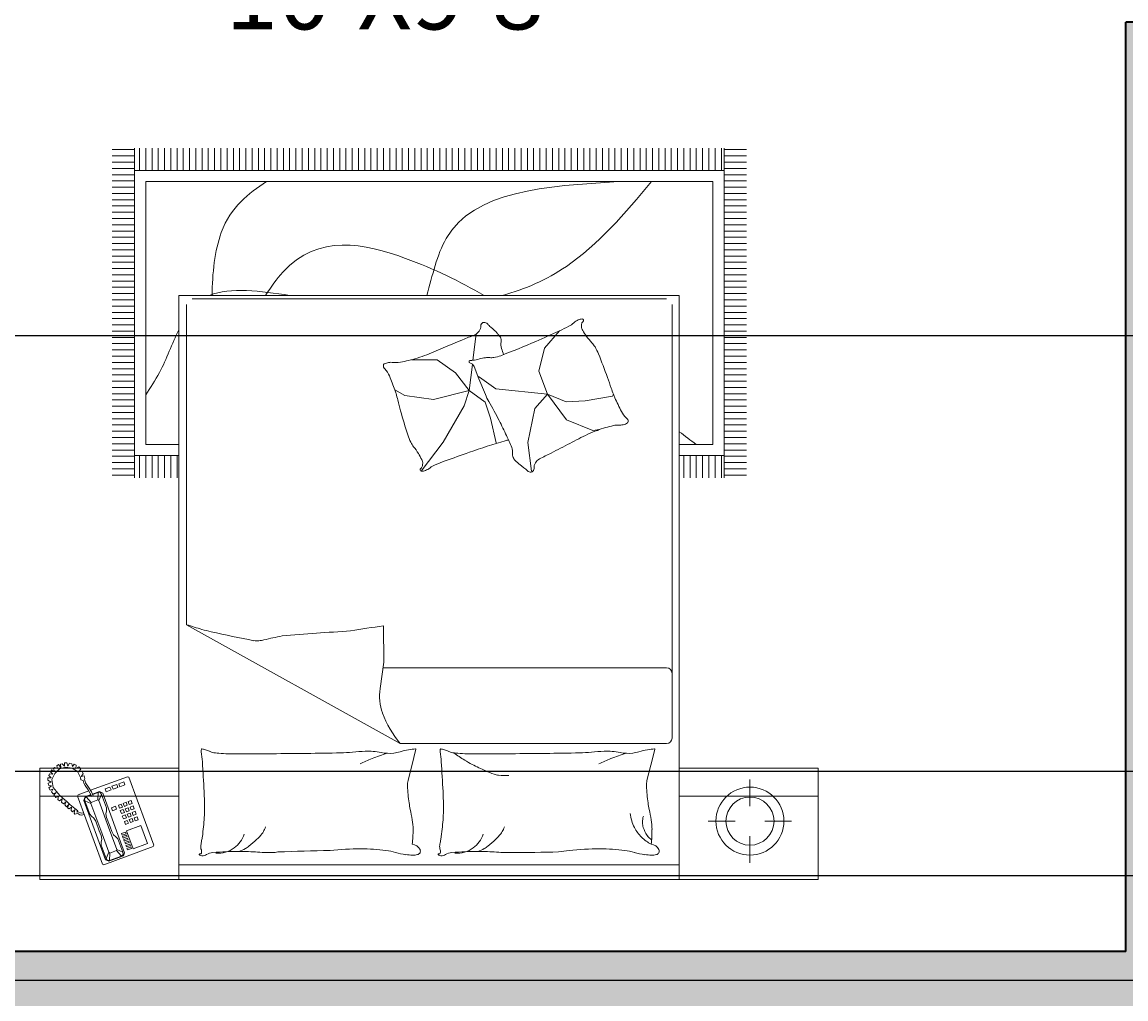
# Model space of a CAD drawing. Units: inches. Extents: x 311 to 815, y -527 to 136.
# Tile 8 of 21: x 444 to 539, y -294 to -210. Entities that reach past the tile are written whole.
import ezdxf

# ---------------------------------------------------------------- set-up
doc = ezdxf.new("R2010")
doc.units = ezdxf.units.IN
doc.header["$MEASUREMENT"] = 0
for name, color, linetype, lineweight in [('A-ANNO-DIMS', 1, 'Continuous', 18), ('A-AREA-IDEN', 8, 'Continuous', 18), ('A-WALL-PATT', 242, 'Continuous', 13), ('wall', 1, 'Continuous', 35)]:
    doc.layers.add(name, color=color, linetype=linetype, lineweight=lineweight)
doc.layers.add('furniture', color=50, linetype='Continuous', lineweight=13, transparency=0.8)
doc.styles.add('DIM_FONT', font='SIMPLEX.shx', dxfattribs={"width": 0.8})
doc.styles.get("Standard").update_dxf_attribs({"font": 'arial.ttf'})
doc.dimstyles.get("Standard").update_dxf_attribs({"dimtxt": 0.18, "dimasz": 0.18, "dimexe": 0.18, "dimexo": 0.0625, "dimgap": 0.09, "dimtad": 0, "dimtih": 1, "dimtoh": 1, "dimdec": 1, "dimzin": 0, "dimdsep": 46, "dimlunit": 4, "dimtxsty": 'Standard', "dimcen": 0.09, "dimadec": 0, "dimazin": 0, "dimtfac": 1, "dimtdec": 1, "dimtofl": 0, "dimtmove": 0, "dimatfit": 3, "dimfxl": 1, "dimtolj": 1, "dimtzin": 0, "dimarcsym": 0})

# ---------------------------------------------------------------- blocks, each defined once
blk = doc.blocks.new('A$C4F634EDD')
for p, q in [((0, 2.6295), (0, 2.2295)), ((0.5, 2.6295), (0, 2.6295)), ((0.5, 2.6295), (2.3, 2.6295)), ((0.5, 0.5295), (0.5, 2.6295)), ((0.5, 2.2295), (0.5, 2.6295)), ((2.3, 2.6295), (2.3, 0.5295)), ((2.3, 2.6295), (2.8, 2.6295)), ((2.3, 2.2295), (2.3, 2.6295)), ((2.8, 2.6295), (2.8, 2.2295)), ((0.2457, 2.5697), (0.2457, 2.4733)), ((0.5, 2.5771), (2.3, 2.5771)), ((2.392, 2.5115), (2.5692, 2.5765)), ((2.4946, 2.5331), (2.4985, 2.5445)), ((2.4985, 2.5445), (2.5516, 2.564)), ((2.5062, 2.5454), (2.5004, 2.5392)), ((2.5062, 2.5454), (2.5487, 2.561)), ((2.5235, 2.5256), (2.5062, 2.5454)), ((2.5483, 2.5347), (2.5487, 2.561)), ((2.5487, 2.561), (2.5571, 2.56)), ((2.5615, 2.5536), (2.5514, 2.5318)), ((2.5516, 2.564), (2.5637, 2.5584)), ((2.5571, 2.56), (2.5615, 2.5536)), ((2.5615, 2.5536), (2.5791, 2.5058)), ((2.5637, 2.5584), (2.6418, 2.3458)), ((2.5692, 2.5765), (2.574, 2.5743)), ((2.574, 2.5743), (2.6638, 2.3298)), ((2.3898, 2.5066), (2.392, 2.5115)), ((2.4795, 2.2621), (2.3898, 2.5066)), ((2.412, 2.5007), (2.4634, 2.5196)), ((2.4634, 2.5196), (2.4875, 2.454)), ((2.4842, 2.5232), (2.47, 2.518)), ((2.47, 2.518), (2.472, 2.5127)), ((2.472, 2.5127), (2.4862, 2.5179)), ((2.4881, 2.5126), (2.4739, 2.5074)), ((2.4739, 2.5074), (2.4759, 2.502)), ((2.4759, 2.502), (2.4901, 2.5073)), ((2.492, 2.5019), (2.4778, 2.4967)), ((2.4862, 2.5179), (2.4842, 2.5232)), ((2.4901, 2.5073), (2.4881, 2.5126)), ((2.494, 2.4966), (2.492, 2.5019)), ((2.5734, 2.3187), (2.4946, 2.5331)), ((2.5004, 2.5392), (2.5013, 2.5315)), ((2.5013, 2.5315), (2.5188, 2.4836)), ((2.5013, 2.5315), (2.5231, 2.5214)), ((2.5231, 2.5214), (2.5235, 2.5256)), ((2.5523, 2.4417), (2.5231, 2.5214)), ((2.5483, 2.5347), (2.5235, 2.5256)), ((2.5514, 2.5318), (2.5483, 2.5347)), ((2.5807, 2.4521), (2.5514, 2.5318)), ((2.5791, 2.5058), (2.5788, 2.4956)), ((2.4361, 2.4352), (2.412, 2.5007)), ((2.4778, 2.4967), (2.4798, 2.4914)), ((2.4798, 2.4914), (2.494, 2.4966)), ((2.4959, 2.4913), (2.4817, 2.4861)), ((2.4817, 2.4861), (2.4837, 2.4808)), ((2.4837, 2.4808), (2.4979, 2.486)), ((2.4998, 2.4807), (2.4856, 2.4755)), ((2.4856, 2.4755), (2.4876, 2.4702)), ((2.4876, 2.4702), (2.5018, 2.4754)), ((2.5037, 2.47), (2.4895, 2.4648)), ((2.4895, 2.4648), (2.4915, 2.4595)), ((2.4915, 2.4595), (2.5057, 2.4647)), ((2.4979, 2.486), (2.4959, 2.4913)), ((2.5018, 2.4754), (2.4998, 2.4807)), ((2.5057, 2.4647), (2.5037, 2.47)), ((2.5188, 2.4836), (2.5256, 2.4761)), ((2.5256, 2.4761), (2.5342, 2.4692)), ((2.5342, 2.4692), (2.5405, 2.4574)), ((2.5788, 2.4956), (2.5767, 2.4848)), ((2.5767, 2.4848), (2.5795, 2.4717)), ((2.5795, 2.4717), (2.586, 2.454)), ((2.4875, 2.454), (2.4361, 2.4352)), ((2.4634, 2.4211), (2.474, 2.425)), ((2.474, 2.425), (2.4779, 2.4143)), ((2.4811, 2.4276), (2.4917, 2.4315)), ((2.485, 2.4169), (2.4811, 2.4276)), ((2.4917, 2.4315), (2.4956, 2.4208)), ((2.5405, 2.4574), (2.547, 2.4397)), ((2.5594, 2.4061), (2.547, 2.4397)), ((2.5523, 2.4417), (2.5875, 2.346)), ((2.5807, 2.4521), (2.6158, 2.3564)), ((2.5984, 2.4204), (2.586, 2.454)), ((0.0957, 2.4197), (0.192, 2.4197)), ((0.2994, 2.4197), (0.3957, 2.4197)), ((2.4457, 2.4146), (2.4563, 2.4185)), ((2.4496, 2.4039), (2.4457, 2.4146)), ((2.4602, 2.4078), (2.4496, 2.4039)), ((2.4528, 2.3951), (2.4635, 2.399)), ((2.4567, 2.3844), (2.4528, 2.3951)), ((2.4563, 2.4185), (2.4602, 2.4078)), ((2.4674, 2.3883), (2.4567, 2.3844)), ((2.4673, 2.4104), (2.4634, 2.4211)), ((2.4635, 2.399), (2.4674, 2.3883)), ((2.4779, 2.4143), (2.4673, 2.4104)), ((2.4706, 2.4016), (2.4812, 2.4055)), ((2.4745, 2.3909), (2.4706, 2.4016)), ((2.4851, 2.3949), (2.4745, 2.3909)), ((2.4777, 2.3821), (2.4883, 2.386)), ((2.4816, 2.3715), (2.4777, 2.3821)), ((2.4812, 2.4055), (2.4851, 2.3949)), ((2.4956, 2.4208), (2.485, 2.4169)), ((2.4883, 2.4081), (2.4989, 2.412)), ((2.4922, 2.3975), (2.4883, 2.4081)), ((2.4883, 2.386), (2.4922, 2.3754)), ((2.5028, 2.4014), (2.4922, 2.3975)), ((2.4954, 2.3886), (2.5061, 2.3925)), ((2.4993, 2.378), (2.4954, 2.3886)), ((2.4989, 2.412), (2.5028, 2.4014)), ((2.51, 2.3819), (2.4993, 2.378)), ((2.5061, 2.3925), (2.51, 2.3819)), ((2.5238, 2.3769), (2.538, 2.3821)), ((2.538, 2.3821), (2.5419, 2.3715)), ((2.5622, 2.393), (2.5594, 2.4061)), ((2.5598, 2.372), (2.5601, 2.3822)), ((2.5601, 2.3822), (2.5622, 2.393)), ((2.6047, 2.4086), (2.5984, 2.4204)), ((2.6133, 2.4017), (2.6047, 2.4086)), ((2.6201, 2.3941), (2.6133, 2.4017)), ((2.6376, 2.3463), (2.6201, 2.3941)), ((2.6499, 2.3979), (2.6397, 2.3953)), ((2.6417, 2.39), (2.6488, 2.391)), ((2.6488, 2.391), (2.6538, 2.3895)), ((2.6551, 2.397), (2.6499, 2.3979)), ((2.6538, 2.3895), (2.6596, 2.388)), ((2.6627, 2.392), (2.6551, 2.397)), ((2.6596, 2.388), (2.6626, 2.3867)), ((2.6626, 2.3867), (2.6662, 2.388)), ((2.6692, 2.394), (2.6627, 2.392)), ((2.6662, 2.388), (2.6632, 2.3828)), ((2.6632, 2.3828), (2.6736, 2.3744)), ((2.6736, 2.3944), (2.6692, 2.394)), ((2.6765, 2.391), (2.6736, 2.3944)), ((2.6742, 2.3795), (2.6765, 2.391)), ((2.6824, 2.3858), (2.6742, 2.3795)), ((2.6873, 2.3815), (2.6824, 2.3858)), ((0.2457, 2.366), (0.2457, 2.2697)), ((2.46, 2.3756), (2.4706, 2.3795)), ((2.4639, 2.365), (2.46, 2.3756)), ((2.4745, 2.3689), (2.4639, 2.365)), ((2.4672, 2.3561), (2.4778, 2.36)), ((2.4711, 2.3455), (2.4672, 2.3561)), ((2.4706, 2.3795), (2.4745, 2.3689)), ((2.4817, 2.3494), (2.4711, 2.3455)), ((2.4778, 2.36), (2.4817, 2.3494)), ((2.4922, 2.3754), (2.4816, 2.3715)), ((2.4849, 2.3626), (2.4955, 2.3665)), ((2.4888, 2.352), (2.4849, 2.3626)), ((2.4994, 2.3559), (2.4888, 2.352)), ((2.4955, 2.3665), (2.4994, 2.3559)), ((2.5026, 2.3691), (2.5132, 2.373)), ((2.5065, 2.3585), (2.5026, 2.3691)), ((2.5171, 2.3624), (2.5065, 2.3585)), ((2.5132, 2.373), (2.5171, 2.3624)), ((2.5277, 2.3663), (2.5238, 2.3769)), ((2.5419, 2.3715), (2.5277, 2.3663)), ((2.5774, 2.3242), (2.5598, 2.372)), ((2.5774, 2.3242), (2.5875, 2.346)), ((2.5875, 2.346), (2.5905, 2.3431)), ((2.5905, 2.3431), (2.5901, 2.3168)), ((2.6154, 2.3522), (2.5905, 2.3431)), ((2.6158, 2.3564), (2.6154, 2.3522)), ((2.6154, 2.3522), (2.6327, 2.3324)), ((2.6376, 2.3463), (2.6158, 2.3564)), ((2.6418, 2.3458), (2.6369, 2.332)), ((2.6385, 2.3386), (2.6376, 2.3463)), ((2.6736, 2.3744), (2.6922, 2.3593)), ((2.6853, 2.369), (2.6873, 2.3815)), ((2.6946, 2.376), (2.6853, 2.369)), ((2.6922, 2.3593), (2.7051, 2.3473)), ((2.6995, 2.3713), (2.6946, 2.376)), ((2.695, 2.3603), (2.6995, 2.3713)), ((2.7031, 2.3682), (2.695, 2.3603)), ((2.7096, 2.3616), (2.7031, 2.3682)), ((2.7051, 2.3473), (2.7079, 2.3475)), ((2.7062, 2.351), (2.7096, 2.3616)), ((2.7147, 2.3578), (2.7062, 2.351)), ((2.7079, 2.3475), (2.7079, 2.3443)), ((2.7079, 2.3443), (2.727, 2.3277)), ((2.7214, 2.3517), (2.7147, 2.3578)), ((2.7196, 2.34), (2.7214, 2.3517)), ((2.7286, 2.3466), (2.7196, 2.34)), ((2.7346, 2.3423), (2.7286, 2.3466)), ((2.732, 2.3295), (2.7346, 2.3423)), ((0, 2.3301), (0.5, 2.3301)), ((2.8, 2.3301), (2.3, 2.3301)), ((2.6172, 2.3086), (2.4844, 2.2599)), ((2.5362, 2.305), (2.5185, 2.2985)), ((2.5401, 2.2944), (2.5362, 2.305)), ((2.561, 2.3141), (2.5433, 2.3076)), ((2.5433, 2.3076), (2.5472, 2.297)), ((2.5472, 2.297), (2.5649, 2.3035)), ((2.5649, 2.3035), (2.561, 2.3141)), ((2.5855, 2.3131), (2.5734, 2.3187)), ((2.5818, 2.3178), (2.5774, 2.3242)), ((2.5901, 2.3168), (2.5818, 2.3178)), ((2.6104, 2.3222), (2.5855, 2.3131)), ((2.5901, 2.3168), (2.6097, 2.324)), ((2.613, 2.3312), (2.6077, 2.3293)), ((2.6077, 2.3293), (2.6135, 2.3141)), ((2.6192, 2.3174), (2.613, 2.3312)), ((2.6135, 2.3141), (2.6244, 2.2977)), ((2.6153, 2.3261), (2.6327, 2.3324)), ((2.6369, 2.332), (2.6161, 2.3243)), ((2.626, 2.3069), (2.6192, 2.3174)), ((2.6616, 2.3249), (2.6234, 2.3109)), ((2.6365, 2.2916), (2.626, 2.3069)), ((2.6327, 2.3324), (2.6385, 2.3386)), ((2.6638, 2.3298), (2.6616, 2.3249)), ((2.727, 2.3277), (2.7512, 2.2983)), ((2.7423, 2.3345), (2.732, 2.3295)), ((2.7406, 2.3172), (2.7495, 2.325)), ((2.7519, 2.3218), (2.7406, 2.3172)), ((2.7495, 2.325), (2.7423, 2.3345)), ((2.7575, 2.3144), (2.7519, 2.3218)), ((2.7526, 2.3045), (2.7575, 2.3144)), ((2.7622, 2.308), (2.7526, 2.3045)), ((2.7673, 2.2997), (2.7622, 2.308)), ((0.5953, 2.1912), (0.616, 2.2738)), ((1.4546, 2.1912), (1.4752, 2.2738)), ((2.5114, 2.2959), (2.4936, 2.2894)), ((2.4936, 2.2894), (2.4976, 2.2788)), ((2.4976, 2.2788), (2.5153, 2.2853)), ((2.5153, 2.2853), (2.5114, 2.2959)), ((2.5185, 2.2985), (2.5224, 2.2879)), ((2.5224, 2.2879), (2.5401, 2.2944)), ((2.6244, 2.2977), (2.6349, 2.2825)), ((2.6349, 2.2825), (2.638, 2.273)), ((2.6407, 2.2834), (2.6365, 2.2916)), ((2.6399, 2.2712), (2.6374, 2.2659)), ((2.6374, 2.2659), (2.6398, 2.257)), ((2.638, 2.273), (2.6399, 2.2712)), ((2.6438, 2.2739), (2.6407, 2.2834)), ((2.6519, 2.2716), (2.6438, 2.2739)), ((2.6535, 2.2628), (2.6519, 2.2716)), ((2.6636, 2.2409), (2.6535, 2.2628)), ((2.756, 2.2695), (2.7459, 2.2483)), ((2.7512, 2.2983), (2.756, 2.2695)), ((2.7574, 2.2924), (2.7673, 2.2997)), ((2.7687, 2.2905), (2.7574, 2.2924)), ((2.7587, 2.279), (2.7699, 2.2828)), ((2.7708, 2.2725), (2.7587, 2.279)), ((2.759, 2.2637), (2.7706, 2.2643)), ((2.7676, 2.2559), (2.759, 2.2637)), ((2.7699, 2.2828), (2.7687, 2.2905)), ((2.7706, 2.2643), (2.7708, 2.2725)), ((0, 2.2295), (0.5, 2.2295)), ((2.8, 2.2295), (2.3, 2.2295)), ((2.4844, 2.2599), (2.4795, 2.2621)), ((2.6398, 2.257), (2.6509, 2.259)), ((2.6509, 2.259), (2.6431, 2.2492)), ((2.6431, 2.2492), (2.6473, 2.2398)), ((2.6473, 2.2398), (2.6592, 2.2429)), ((2.6592, 2.2429), (2.6521, 2.2314)), ((2.6521, 2.2314), (2.6598, 2.2248)), ((2.6598, 2.2248), (2.6697, 2.2309)), ((2.6836, 2.2287), (2.6636, 2.2409)), ((2.6697, 2.2309), (2.6684, 2.219)), ((2.6761, 2.2145), (2.6821, 2.2237)), ((2.6821, 2.2237), (2.6843, 2.2135)), ((2.7063, 2.2256), (2.6836, 2.2287)), ((2.7284, 2.2317), (2.7063, 2.2256)), ((2.7255, 2.2152), (2.7242, 2.2265)), ((2.7242, 2.2265), (2.7324, 2.2165)), ((2.7459, 2.2483), (2.7284, 2.2317)), ((2.7386, 2.2208), (2.7354, 2.2306)), ((2.7354, 2.2306), (2.7462, 2.2264)), ((2.7509, 2.2314), (2.7459, 2.2418)), ((2.7459, 2.2418), (2.7568, 2.2352)), ((2.7462, 2.2264), (2.7509, 2.2314)), ((2.7529, 2.2505), (2.7645, 2.2498)), ((2.7607, 2.2424), (2.7529, 2.2505)), ((2.7568, 2.2352), (2.7607, 2.2424)), ((2.7645, 2.2498), (2.7676, 2.2559)), ((0.5878, 2.1612), (0.5953, 2.1912)), ((1.4471, 2.1612), (1.4546, 2.1912)), ((2.6684, 2.219), (2.6761, 2.2145)), ((2.6843, 2.2135), (2.6927, 2.2117)), ((2.6927, 2.2117), (2.6986, 2.222)), ((2.6986, 2.222), (2.7019, 2.2098)), ((2.7019, 2.2098), (2.7102, 2.2104)), ((2.7102, 2.2104), (2.7113, 2.2218)), ((2.7113, 2.2218), (2.7192, 2.2137)), ((2.7192, 2.2137), (2.7255, 2.2152)), ((2.7324, 2.2165), (2.7386, 2.2208)), ((0.5258, 2.121), (0.5258, 0.5617)), ((1.5035, 2.141), (0.5458, 2.141)), ((1.5035, 2.141), (2.2716, 1.7136)), ((1.576, 1.9433), (1.5624, 1.8479)), ((0.5458, 1.8684), (1.5653, 1.8684)), ((1.5624, 1.8479), (1.5641, 1.7178)), ((2.2716, 0.5617), (2.2716, 1.7136)), ((0.2586, 1.1753), (0.3386, 1.1753)), ((0.2586, 1.1528), (0.3386, 1.1528)), ((0.3386, 0), (0.3386, 1.1852)), ((0.3486, 1.1052), (0.3486, 1.1852)), ((0.3711, 1.1052), (0.3711, 1.1852)), ((0.3936, 1.1052), (0.3936, 1.1852)), ((0.4161, 1.1052), (0.4161, 1.1852)), ((0.4386, 1.1052), (0.4386, 1.1852)), ((0.4611, 1.1052), (0.4611, 1.1852)), ((0.4836, 1.1052), (0.4836, 1.1852)), ((1.031, 1.1612), (1.0448, 1.0581)), ((1.4276, 1.1611), (1.3484, 1.0571)), ((2.3061, 1.1052), (2.3061, 1.1852)), ((2.3286, 1.1052), (2.3286, 1.1852)), ((2.3511, 1.1052), (2.3511, 1.1852)), ((2.3736, 1.1052), (2.3736, 1.1852)), ((2.3961, 1.1052), (2.3961, 1.1852)), ((2.4186, 1.1052), (2.4186, 1.1852)), ((2.4411, 1.1052), (2.4411, 1.1852)), ((2.4588, 1.1852), (2.4588, 0)), ((2.4588, 1.1753), (2.5388, 1.1753)), ((2.4588, 1.1528), (2.5388, 1.1528)), ((0.2586, 1.1303), (0.3386, 1.1303)), ((2.4588, 1.1303), (2.5388, 1.1303)), ((0.2586, 1.1078), (0.3386, 1.1078)), ((0.2586, 1.0853), (0.3386, 1.0853)), ((0.3386, 1.1052), (0.5, 1.1052)), ((2.3, 1.1052), (2.4588, 1.1052)), ((2.4588, 1.1078), (2.5388, 1.1078)), ((2.4588, 1.0853), (2.5388, 1.0853)), ((0.2586, 1.0628), (0.3386, 1.0628)), ((0.2586, 1.0403), (0.3386, 1.0403)), ((0.3786, 1.0652), (0.5, 1.0652)), ((0.3786, 0.12), (0.3786, 1.0652)), ((1.0448, 1.0581), (1.019, 0.936)), ((1.1784, 0.9702), (1.1586, 1.0591)), ((1.3484, 1.0571), (1.2733, 0.9268)), ((2.3, 1.0652), (2.4188, 1.0652)), ((2.4188, 1.0652), (2.4188, 0.12)), ((2.4588, 1.0628), (2.5388, 1.0628)), ((2.4588, 1.0403), (2.5388, 1.0403)), ((0.2586, 1.0178), (0.3386, 1.0178)), ((0.2586, 0.9953), (0.3386, 0.9953)), ((0.8108, 1.0151), (0.7868, 1.0117)), ((0.9054, 0.9773), (0.8108, 1.0151)), ((2.4588, 1.0178), (2.5388, 1.0178)), ((2.4588, 0.9953), (2.5388, 0.9953)), ((0.2586, 0.9728), (0.3386, 0.9728)), ((0.9743, 0.8845), (0.9054, 0.9773)), ((1.1982, 0.9129), (1.1784, 0.9702)), ((2.4588, 0.9728), (2.5388, 0.9728)), ((0.2586, 0.9503), (0.3386, 0.9503)), ((0.2586, 0.9278), (0.3386, 0.9278)), ((1.019, 0.936), (0.9743, 0.8845)), ((1.2733, 0.9268), (1.2555, 0.8715)), ((2.4588, 0.9503), (2.5388, 0.9503)), ((2.4588, 0.9278), (2.5388, 0.9278)), ((0.2586, 0.9053), (0.3386, 0.9053)), ((0.2586, 0.8828), (0.3386, 0.8828)), ((0.7403, 0.8913), (0.737, 0.8849)), ((0.8384, 0.9085), (0.7403, 0.8913)), ((0.9072, 0.912), (0.8384, 0.9085)), ((0.9743, 0.8845), (0.9072, 0.912)), ((0.9743, 0.8845), (1.0052, 0.802)), ((0.9743, 0.8845), (1.16, 0.8656)), ((1.1973, 0.8853), (1.2203, 0.829)), ((1.2555, 0.8715), (1.1982, 0.9129)), ((1.2555, 0.8715), (1.384, 0.9031)), ((1.384, 0.9031), (1.4868, 0.8892)), ((1.4868, 0.8892), (1.5228, 0.8692)), ((2.4588, 0.9053), (2.5388, 0.9053)), ((2.4588, 0.8828), (2.5388, 0.8828)), ((0.2586, 0.8603), (0.3386, 0.8603)), ((0.2586, 0.8378), (0.3386, 0.8378)), ((1.16, 0.8656), (1.2099, 0.8295)), ((1.2555, 0.8715), (1.2437, 0.7773)), ((1.2555, 0.8715), (1.3049, 0.8082)), ((2.4588, 0.8603), (2.5388, 0.8603)), ((2.4588, 0.8378), (2.5388, 0.8378)), ((0.2586, 0.8153), (0.3386, 0.8153)), ((1.0052, 0.802), (0.9846, 0.7194)), ((1.2099, 0.8295), (1.222, 0.8209)), ((1.2203, 0.829), (1.2381, 0.7855)), ((1.3049, 0.8082), (1.3701, 0.7608)), ((2.4588, 0.8153), (2.5388, 0.8153)), ((0.2586, 0.7928), (0.3386, 0.7928)), ((0.2586, 0.7703), (0.3386, 0.7703)), ((1.2419, 0.7626), (1.23, 0.668)), ((1.3701, 0.7608), (1.463, 0.7608)), ((2.4588, 0.7928), (2.5388, 0.7928)), ((2.4588, 0.7703), (2.5388, 0.7703)), ((0.2586, 0.7478), (0.3386, 0.7478)), ((0.2586, 0.7253), (0.3386, 0.7253)), ((0.9846, 0.7194), (0.931, 0.6569)), ((2.4588, 0.7478), (2.5388, 0.7478)), ((2.4588, 0.7253), (2.5388, 0.7253)), ((0.2586, 0.7028), (0.3386, 0.7028)), ((0.2586, 0.6803), (0.3386, 0.6803)), ((2.4588, 0.7028), (2.5388, 0.7028)), ((2.4588, 0.6803), (2.5388, 0.6803)), ((0.2586, 0.6578), (0.3386, 0.6578)), ((0.2586, 0.6353), (0.3386, 0.6353)), ((2.4588, 0.6578), (2.5388, 0.6578)), ((2.4588, 0.6353), (2.5388, 0.6353)), ((0.2586, 0.6128), (0.3386, 0.6128)), ((2.4588, 0.6128), (2.5388, 0.6128)), ((0.2586, 0.5903), (0.3386, 0.5903)), ((0.2586, 0.5678), (0.3386, 0.5678)), ((2.4588, 0.5903), (2.5388, 0.5903)), ((2.4588, 0.5678), (2.5388, 0.5678)), ((0.2586, 0.5453), (0.3386, 0.5453)), ((0.2586, 0.5228), (0.3386, 0.5228)), ((2.3, 0.5295), (0.5, 0.5295)), ((0.5458, 0.5417), (2.2516, 0.5417)), ((2.4588, 0.5453), (2.5388, 0.5453)), ((2.4588, 0.5228), (2.5388, 0.5228)), ((0.2586, 0.5003), (0.3386, 0.5003)), ((0.2586, 0.4778), (0.3386, 0.4778)), ((2.4588, 0.5003), (2.5388, 0.5003)), ((2.4588, 0.4778), (2.5388, 0.4778)), ((0.2586, 0.4553), (0.3386, 0.4553)), ((2.4588, 0.4553), (2.5388, 0.4553)), ((0.2586, 0.4328), (0.3386, 0.4328)), ((0.2586, 0.4103), (0.3386, 0.4103)), ((2.4588, 0.4328), (2.5388, 0.4328)), ((2.4588, 0.4103), (2.5388, 0.4103)), ((0.2586, 0.3878), (0.3386, 0.3878)), ((0.2586, 0.3653), (0.3386, 0.3653)), ((2.4588, 0.3878), (2.5388, 0.3878)), ((2.4588, 0.3653), (2.5388, 0.3653)), ((0.2586, 0.3428), (0.3386, 0.3428)), ((0.2586, 0.3203), (0.3386, 0.3203)), ((2.4588, 0.3428), (2.5388, 0.3428)), ((2.4588, 0.3203), (2.5388, 0.3203)), ((0.2586, 0.2978), (0.3386, 0.2978)), ((2.4588, 0.2978), (2.5388, 0.2978)), ((0.2586, 0.2753), (0.3386, 0.2753)), ((0.2586, 0.2528), (0.3386, 0.2528)), ((2.4588, 0.2753), (2.5388, 0.2753)), ((2.4588, 0.2528), (2.5388, 0.2528)), ((0.2586, 0.2303), (0.3386, 0.2303)), ((0.2586, 0.2078), (0.3386, 0.2078)), ((2.4588, 0.2303), (2.5388, 0.2303)), ((2.4588, 0.2078), (2.5388, 0.2078)), ((0.2586, 0.1853), (0.3386, 0.1853)), ((0.2586, 0.1628), (0.3386, 0.1628)), ((2.4588, 0.1853), (2.5388, 0.1853)), ((2.4588, 0.1628), (2.5388, 0.1628)), ((0.2586, 0.1403), (0.3386, 0.1403)), ((2.4188, 0.12), (0.3786, 0.12)), ((2.4588, 0.1403), (2.5388, 0.1403)), ((0.2586, 0.1178), (0.3386, 0.1178)), ((0.2586, 0.0953), (0.3386, 0.0953)), ((2.4588, 0.08), (0.3386, 0.08)), ((0.3486, 0), (0.3486, 0.08)), ((0.3711, 0), (0.3711, 0.08)), ((0.3936, 0), (0.3936, 0.08)), ((0.4161, 0), (0.4161, 0.08)), ((0.4386, 0), (0.4386, 0.08)), ((0.4611, 0), (0.4611, 0.08)), ((0.4836, 0), (0.4836, 0.08)), ((0.5061, 0), (0.5061, 0.08)), ((0.5286, 0), (0.5286, 0.08)), ((0.5511, 0), (0.5511, 0.08)), ((0.5736, 0), (0.5736, 0.08)), ((0.5961, 0), (0.5961, 0.08)), ((0.6186, 0), (0.6186, 0.08)), ((0.6411, 0), (0.6411, 0.08)), ((0.6636, 0), (0.6636, 0.08)), ((0.6861, 0), (0.6861, 0.08)), ((0.7086, 0), (0.7086, 0.08)), ((0.7311, 0), (0.7311, 0.08)), ((0.7536, 0), (0.7536, 0.08)), ((0.7761, 0), (0.7761, 0.08)), ((0.7986, 0), (0.7986, 0.08)), ((0.8211, 0), (0.8211, 0.08)), ((0.8436, 0), (0.8436, 0.08)), ((0.8661, 0), (0.8661, 0.08)), ((0.8886, 0), (0.8886, 0.08)), ((0.9111, 0), (0.9111, 0.08)), ((0.9336, 0), (0.9336, 0.08)), ((0.9561, 0), (0.9561, 0.08)), ((0.9786, 0), (0.9786, 0.08)), ((1.0011, 0), (1.0011, 0.08)), ((1.0236, 0), (1.0236, 0.08)), ((1.0461, 0), (1.0461, 0.08)), ((1.0686, 0), (1.0686, 0.08)), ((1.0911, 0), (1.0911, 0.08)), ((1.1136, 0), (1.1136, 0.08)), ((1.1361, 0), (1.1361, 0.08)), ((1.1586, 0), (1.1586, 0.08)), ((1.1811, 0), (1.1811, 0.08)), ((1.2036, 0), (1.2036, 0.08)), ((1.2261, 0), (1.2261, 0.08)), ((1.2486, 0), (1.2486, 0.08)), ((1.2711, 0), (1.2711, 0.08)), ((1.2936, 0), (1.2936, 0.08)), ((1.3161, 0), (1.3161, 0.08)), ((1.3386, 0), (1.3386, 0.08)), ((1.3611, 0), (1.3611, 0.08)), ((1.3836, 0), (1.3836, 0.08)), ((1.4061, 0), (1.4061, 0.08)), ((1.4286, 0), (1.4286, 0.08)), ((1.4511, 0), (1.4511, 0.08)), ((1.4736, 0), (1.4736, 0.08)), ((1.4961, 0), (1.4961, 0.08)), ((1.5186, 0), (1.5186, 0.08)), ((1.5411, 0), (1.5411, 0.08)), ((1.5636, 0), (1.5636, 0.08)), ((1.5861, 0), (1.5861, 0.08)), ((1.6086, 0), (1.6086, 0.08)), ((1.6311, 0), (1.6311, 0.08)), ((1.6536, 0), (1.6536, 0.08)), ((1.6761, 0), (1.6761, 0.08)), ((1.6986, 0), (1.6986, 0.08)), ((1.7211, 0), (1.7211, 0.08)), ((1.7436, 0), (1.7436, 0.08)), ((1.7661, 0), (1.7661, 0.08)), ((1.7886, 0), (1.7886, 0.08)), ((1.8111, 0), (1.8111, 0.08)), ((1.8336, 0), (1.8336, 0.08)), ((1.8561, 0), (1.8561, 0.08)), ((1.8786, 0), (1.8786, 0.08)), ((1.9011, 0), (1.9011, 0.08)), ((1.9236, 0), (1.9236, 0.08)), ((1.9461, 0), (1.9461, 0.08)), ((1.9686, 0), (1.9686, 0.08)), ((1.9911, 0), (1.9911, 0.08)), ((2.0136, 0), (2.0136, 0.08)), ((2.0361, 0), (2.0361, 0.08)), ((2.0586, 0), (2.0586, 0.08)), ((2.0811, 0), (2.0811, 0.08)), ((2.1036, 0), (2.1036, 0.08)), ((2.1261, 0), (2.1261, 0.08)), ((2.1486, 0), (2.1486, 0.08)), ((2.1711, 0), (2.1711, 0.08)), ((2.1936, 0), (2.1936, 0.08)), ((2.2161, 0), (2.2161, 0.08)), ((2.2386, 0), (2.2386, 0.08)), ((2.2611, 0), (2.2611, 0.08)), ((2.2836, 0), (2.2836, 0.08)), ((2.3061, 0), (2.3061, 0.08)), ((2.3286, 0), (2.3286, 0.08)), ((2.3511, 0), (2.3511, 0.08)), ((2.3736, 0), (2.3736, 0.08)), ((2.3961, 0), (2.3961, 0.08)), ((2.4186, 0), (2.4186, 0.08)), ((2.4411, 0), (2.4411, 0.08)), ((2.4588, 0.1178), (2.5388, 0.1178)), ((2.4588, 0.0953), (2.5388, 0.0953)), ((0.2586, 0.0728), (0.3386, 0.0728)), ((0.2586, 0.0503), (0.3386, 0.0503)), ((2.4588, 0.0728), (2.5388, 0.0728)), ((2.4588, 0.0503), (2.5388, 0.0503)), ((0.2586, 0.0278), (0.3386, 0.0278)), ((0.2586, 0.0053), (0.3386, 0.0053)), ((2.4588, 0.0278), (2.5388, 0.0278)), ((2.4588, 0.0053), (2.5388, 0.0053))]:
    blk.add_line(p, q)
for radius in [0.1222, 0.0865]:
    blk.add_circle((0.2457, 2.4197), radius)
for centre, radius, start, end in [((0.5999, 2.4516), 0.0904, 90, 101.2724), ((0.5999, 2.3808), 0.1611, 81.5628, 90), ((1.3554, 2.5152), 0.0289, 85.6975, 120.6513), ((1.3556, 2.519), 0.0251, 68.2117, 85.6975), ((1.3637, 2.5391), 0.00342, 19.564, 68.2117), ((1.4591, 2.4516), 0.0904, 90, 101.2724), ((1.4591, 2.3808), 0.1611, 81.5628, 90), ((2.2146, 2.5152), 0.0289, 85.6975, 120.6513), ((2.2149, 2.519), 0.0251, 68.2117, 85.6975), ((2.2229, 2.5391), 0.00342, 19.564, 68.2117), ((0.5848, 2.5274), 0.0131, 101.2724, 206.5805), ((0.6036, 2.5368), 0.0342, 206.5805, 265.5998), ((1.0898, 2.4496), 0.4918, 173.7676, 180), ((0.5368, 2.3783), 0.1399, 45.0976, 62.7964), ((0.5788, 2.2388), 0.3048, 74.256, 81.5628), ((0.7272, 2.7653), 0.2422, 254.256, 262.4531), ((0.7851, 3.2019), 0.6827, 262.4531, 270), ((0.7851, 3.5682), 1.049, 270, 276.0867), ((0.8402, 3.0514), 0.5293, 276.0867, 280.1899), ((1.1602, -8.1346), 10.6675, 90.30153, 91.21582), ((1.1169, 2.2433), 0.2897, 85.1982, 92.5386), ((1.2142, 3.4021), 0.8732, 265.1982, 269.4243), ((1.4317, 2.2032), 0.3916, 128.3886, 133.8115), ((1.2362, 2.45), 0.0768, 117.2396, 128.3886), ((1.3082, 2.3102), 0.234, 110.8603, 117.2396), ((1.2204, 4.0232), 1.4943, 269.4243, 271.9079), ((1.2995, 2.4357), 0.0992, 126.0864, 143.8234), ((1.2995, 2.4357), 0.0992, 105.9352, 126.0864), ((1.2429, 3.3501), 0.8208, 271.9079, 275.2592), ((1.2995, 2.4357), 0.0992, 85.7841, 105.9352), ((1.3132, 2.5864), 0.0539, 275.2592, 300.6513), ((1.3739, 2.5288), 0.0156, 158.0096, 201.421), ((1.1177, 2.5413), 0.246, 347.8905, 351.8665), ((1.3634, 2.533), 0.00428, 78.1069, 158.0096), ((1.3288, 2.5111), 0.0328, 351.8665, 21.421), ((1.3647, 2.5395), 0.00232, 258.1069, 19.564), ((1.444, 2.5274), 0.0131, 101.2724, 206.5805), ((1.4628, 2.5368), 0.0342, 206.5805, 265.5998), ((1.949, 2.4496), 0.4918, 173.7676, 180), ((1.438, 2.2388), 0.3048, 74.256, 81.5628), ((1.5865, 2.7653), 0.2422, 254.256, 262.4531), ((1.6443, 3.2019), 0.6827, 262.4531, 270), ((1.6443, 3.5682), 1.049, 270, 276.0867), ((1.4785, 15.4878), 12.9656, 271.22425, 272.05324), ((1.97, 2.3805), 0.1524, 92.5386, 100.1899), ((1.9761, 2.2433), 0.2897, 85.1982, 92.5386), ((2.0734, 3.4021), 0.8732, 265.1982, 269.4243), ((2.291, 2.2032), 0.3916, 128.3886, 133.8115), ((2.0954, 2.45), 0.0768, 117.2396, 128.3886), ((2.1674, 2.3102), 0.234, 110.8603, 117.2396), ((2.0797, 4.0232), 1.4943, 269.4243, 271.9079), ((2.1588, 2.4357), 0.0992, 126.0864, 143.8234), ((2.1588, 2.4357), 0.0992, 105.9352, 126.0864), ((2.1021, 3.3501), 0.8208, 271.9079, 275.2592), ((2.1588, 2.4357), 0.0992, 85.7841, 105.9352), ((2.1724, 2.5864), 0.0539, 275.2592, 300.6513), ((2.2331, 2.5288), 0.0156, 158.0096, 201.421), ((1.977, 2.5413), 0.246, 347.8905, 351.8665), ((2.2226, 2.533), 0.00428, 78.1069, 158.0096), ((2.1881, 2.5111), 0.0328, 351.8665, 21.421), ((2.224, 2.5395), 0.00232, 258.1069, 19.564), ((0.5462, 2.4142), 0.0899, 41.4429, 53.7359), ((0.5741, 2.4389), 0.0526, 25.3551, 41.4429), ((0.4851, 2.3967), 0.1511, 21.8149, 25.3551), ((0.5368, 2.3783), 0.1399, 27.3988, 45.0976), ((1.1799, 2.4341), 0.0493, 140.9651, 151.6832), ((1.3165, 2.3233), 0.2252, 133.8115, 140.9651), ((1.2995, 2.4357), 0.0992, 143.8234, 161.5603), ((2.2605, 2.3525), 0.9131, 172.3191, 176.6313), ((1.5522, 2.448), 0.1983, 167.8905, 172.3191), ((2.0391, 2.4341), 0.0493, 140.9651, 151.6832), ((2.1757, 2.3233), 0.2252, 133.8115, 140.9651), ((2.1588, 2.4357), 0.0992, 143.8234, 161.5603), ((3.1198, 2.3525), 0.9131, 172.3191, 176.6313), ((2.4114, 2.448), 0.1983, 167.8905, 172.3191), ((0.8019, 2.4496), 0.204, 180, 189.6844), ((0.4345, 2.3765), 0.2056, 18.7799, 21.8149), ((0.576, 2.4246), 0.0562, 0, 18.7799), ((0.5406, 2.4246), 0.0915, 345.3149, 0), ((0.5368, 2.3783), 0.1399, 16.515, 27.3988), ((1.3127, 2.3625), 0.2002, 151.6832, 156.9972), ((1.6611, 2.4496), 0.204, 180, 189.6844), ((2.1719, 2.3625), 0.2002, 151.6832, 156.9972), ((1.4703, 2.5637), 0.882, 189.6844, 192.1984), ((0.5368, 2.3783), 0.1399, 5.6311, 16.515), ((2.0266, 2.3663), 0.6787, 176.6313, 181.6331), ((2.3295, 2.5637), 0.882, 189.6844, 192.1984), ((2.8858, 2.3663), 0.6787, 176.6313, 181.6331), ((0.2982, 2.3103), 0.3171, 8.0051, 12.1984), ((-0.0401, 2.2627), 0.6588, 2.6649, 8.0051), ((2.7128, 2.3859), 1.3652, 181.6331, 183.055), ((1.1575, 2.3103), 0.3171, 8.0051, 12.1984), ((0.8191, 2.2627), 0.6588, 2.6649, 8.0051), ((3.5721, 2.3859), 1.3652, 181.6331, 183.055), ((14.9657, 3.0398), 13.6356, 183.05496, 183.50486), ((15.8249, 3.0398), 13.6356, 183.05496, 183.50486), ((0.5503, 2.2902), 0.0677, 345.9548, 2.6649), ((1.4096, 2.2902), 0.0677, 345.9548, 2.6649), ((1.1303, 1.9835), 0.2721, 85.9172, 93.5552), ((1.1455, 2.197), 0.058, 69.3257, 85.9172), ((0.9871, 1.7772), 0.5066, 65.6735, 69.3257), ((0.6058, 0.9338), 1.4323, 63.5015, 65.6735), ((0.473, 2.8815), 0.7387, 287.1982, 289.428), ((0.473, 2.8815), 0.7387, 289.428, 291.6577), ((0.473, 2.8815), 0.7387, 291.6577, 293.4844), ((0.473, 2.8815), 0.7387, 293.4844, 295.3111), ((1.1054, 1.9358), 0.3126, 57.865, 63.5015), ((0.8841, 1.5835), 0.7286, 54.1737, 57.865), ((1.6762, 2.2258), 0.3212, 183.5049, 189.9984), ((1.3322, 2.8815), 0.7387, 287.1982, 289.428), ((1.3322, 2.8815), 0.7387, 289.428, 291.6577), ((1.3322, 2.8815), 0.7387, 291.6577, 293.4844), ((1.3322, 2.8815), 0.7387, 293.4844, 295.3111), ((2.5355, 2.2258), 0.3212, 183.5049, 189.9984), ((0.5887, 2.1609), 0.000917, 165.9551, 274.0829), ((0.5695, 2.4301), 0.2708, 274.0829, 279.4841), ((0.5763, 2.3896), 0.2297, 279.4841, 287.3864), ((0.6807, 2.0561), 0.1197, 96.4341, 107.3864), ((0.6836, 2.0301), 0.1459, 78.4414, 96.4341), ((0.759, 2.3985), 0.2301, 258.4414, 272.7491), ((0.7026, 3.5718), 1.4048, 272.7491, 274.6176), ((0.9136, 0.9591), 1.2165, 92.6096, 94.6176), ((1.2501, -19.8405), 22.0183, 90.37908, 91.01965), ((1.2012, -3.5404), 5.7185, 89.7135, 90.9704), ((1.224, 1.0141), 1.164, 86.426, 89.7135), ((1.2875, 2.0302), 0.1459, 77.131, 86.426), ((1.3099, 2.1283), 0.0453, 62.7159, 77.131), ((1.3658, 2.2367), 0.0767, 242.7159, 253.7788), ((1.3688, 2.247), 0.0875, 253.7788, 262.8796), ((1.3581, 2.1615), 0.00132, 262.8796, 343.3022), ((1.3409, 2.1667), 0.0193, 343.3022, 9.9984), ((1.448, 2.1609), 0.000917, 165.9551, 274.0829), ((1.4288, 2.4301), 0.2708, 274.0829, 279.4841), ((1.4355, 2.3896), 0.2297, 279.4841, 287.3864), ((1.5399, 2.0561), 0.1197, 96.4341, 107.3864), ((1.5429, 2.0301), 0.1459, 78.4414, 96.4341), ((1.6182, 2.3985), 0.2301, 258.4414, 272.7491), ((1.5619, 3.5718), 1.4048, 272.7491, 274.6176), ((1.7729, 0.9591), 1.2165, 92.6096, 94.6176), ((2.1093, -19.8405), 22.0183, 90.37908, 91.01965), ((2.0605, -3.5404), 5.7185, 89.7135, 90.9704), ((2.0833, 1.0141), 1.164, 86.426, 89.7135), ((2.1467, 2.0302), 0.1459, 77.131, 86.426), ((2.1691, 2.1283), 0.0453, 62.7159, 77.131), ((2.2251, 2.2367), 0.0767, 242.7159, 253.7788), ((2.2281, 2.247), 0.0875, 253.7788, 262.8796), ((2.2174, 2.1615), 0.00132, 262.8796, 343.3022), ((2.2001, 2.1667), 0.0193, 343.3022, 9.9984), ((0.5458, 2.121), 0.02, 90, 180), ((1.2147, 1.9017), 0.3751, 20.1488, 39.6445), ((1.3977, 1.9688), 0.1801, 351.8644, 20.1488), ((0.5458, 1.8884), 0.02, 180, 270), ((0.6102, 18.0525), 16.3521, 273.75703, 274.62393), ((1.4194, 4.2174), 2.5158, 281.6741, 283.1904), ((2.0378, 1.5789), 0.1942, 97.7304, 103.1904), ((2.0195, 1.7137), 0.0581, 79.2724, 97.7304), ((1.2737, -2.2227), 4.0646, 77.0745, 79.2724), ((1.0582, 5.4638), 3.7801, 277.692, 279.495), ((2.0359, 1.0981), 0.6574, 74.0648, 77.0745), ((1.7125, -0.0344), 1.8351, 72.2636, 74.0648), ((0.9863, 1.1494), 0.0359, 297.2902, 3.2455), ((1.0348, 1.1521), 0.0127, 51.1864, 183.2455), ((0.9991, 1.1077), 0.0697, 45.8726, 51.1864), ((1.0791, 1.1902), 0.0452, 225.8726, 232.4713), ((1.2846, 1.4577), 0.3825, 232.4713, 233.7837), ((1.4338, 1.1026), 0.0601, 110.3452, 128.5854), ((1.4251, 1.1259), 0.0352, 86.0516, 110.3452), ((1.4273, 1.1567), 0.00443, 13.2808, 86.0516), ((1.4254, 1.1562), 0.0063, 306.5792, 13.2808), ((-0.4173, 3.8699), 3.0972, 296.4147, 297.2902), ((0.6683, 0.6162), 0.6605, 52.7849, 53.7837), ((0.9362, 0.9689), 0.2176, 46.4776, 52.7849), ((1.0327, 1.0706), 0.0774, 35.8936, 46.4776), ((1.0771, 1.1027), 0.0226, 351.9508, 35.8936), ((-0.4107, 5.9078), 5.0942, 289.0836, 290.1287), ((1.0543, 1.9106), 0.8371, 290.1287, 292.7069), ((1.3469, 1.2115), 0.0792, 292.7069, 308.5854), ((1.4996, 1.1284), 0.0771, 169.5926, 177.2714), ((1.4378, 1.1314), 0.0153, 177.2714, 194.5709), ((1.4611, 1.1374), 0.0393, 194.5709, 206.8179), ((1.4376, 1.1398), 0.0142, 126.5792, 169.5926), ((1.7401, 1.2785), 0.352, 206.8179, 210.9056), ((3.744, -4.3336), 6.1019, 117.49986, 117.84822), ((1.8575, -0.7096), 2.0162, 116.4147, 117.4999), ((1.1449, 1.0931), 0.0458, 171.9508, 202.4162), ((2.032, 1.4591), 1.0054, 202.4162, 205.0529), ((0.2266, 4.0657), 3.145, 286.6085, 289.0836), ((1.6045, 1.1973), 0.194, 210.9056, 219.7005), ((1.3929, 1.0217), 0.081, 26.0735, 39.7005), ((0.5736, 1.5979), 0.6236, 290.7486, 297.4921), ((-1.8336, 6.2238), 5.8383, 297.49208, 297.84822), ((1.0922, 1.1636), 0.1166, 280.7366, 286.6085), ((2.6493, 1.7476), 1.6868, 205.0529, 207.0884), ((1.2892, 0.9709), 0.1965, 17.8396, 26.0735), ((0.7131, 0.9448), 0.0509, 103.0402, 121.6917), ((0.7152, 0.9361), 0.0599, 86.6119, 103.0402), ((0.7224, 1.0587), 0.063, 266.6119, 282.6252), ((0.6422, 1.4168), 0.43, 282.6252, 290.7486), ((-0.4304, 0.4175), 2.003, 15.2625, 17.8396), ((0.6894, 0.9832), 0.0058, 121.6917, 179.0386), ((0.7004, 0.983), 0.0168, 179.0386, 229.4914), ((0.6405, 0.9128), 0.0755, 26.3332, 49.4914), ((2.541, 1.6922), 1.5652, 207.0884, 209.936), ((-1.6775, -0.2344), 2.6619, 25.1732, 26.3332), ((-0.0881, 0.5109), 1.6481, 13.841, 15.2625), ((0.5689, 0.8213), 0.1798, 20.7081, 25.1732), ((0.2268, 0.692), 0.5454, 18.2369, 20.7081), ((0.9989, 0.8042), 0.2143, 22.2355, 29.936), ((2.0418, 1.0357), 0.5454, 193.841, 196.3122), ((1.6908, 0.933), 0.1798, 196.3122, 200.7773), ((2.3102, 1.3785), 1.6481, 198.2369, 199.6584), ((4.0115, 1.8135), 2.6619, 200.7773, 201.9373), ((2.6444, 1.4979), 2.003, 199.6584, 202.2355), ((1.6124, 0.8472), 0.0755, 201.9373, 225.0955), ((1.1727, 0.9313), 0.1794, 277.6784, 284.8807), ((1.2689, 0.569), 0.1955, 97.9822, 104.8807), ((1.2594, 0.7942), 0.0231, 202.2355, 252.8133), ((1.2465, 0.729), 0.034, 85.7407, 97.9822), ((1.2497, 0.772), 0.0092, 265.7407, 289.3799), ((1.2512, 0.7678), 0.00467, 289.3799, 72.8133), ((1.6266, 0.159), 0.6236, 106.3527, 113.0962), ((1.5721, 0.3449), 0.43, 98.2293, 106.3527), ((1.5195, 0.708), 0.063, 82.216, 98.2293), ((1.5362, 0.8298), 0.0599, 262.216, 278.6443), ((1.5375, 0.8209), 0.0509, 278.6443, 297.2959), ((1.5473, 0.7819), 0.0168, 354.6428, 45.0955), ((1.5582, 0.7808), 0.0058, 297.2959, 354.6428), ((0.9722, 0.8143), 0.1965, 202.2355, 210.4694), ((0.8727, 0.7557), 0.081, 210.4694, 224.0964), ((2.2689, -2.1899), 3.145, 111.0043, 113.4795), ((0.1831, 0.4093), 1.0054, 18.0203, 19.3448), ((1.0957, 0.7061), 0.0458, 347.5549, 18.0203), ((1.1834, 0.6373), 0.1166, 98.1216, 111.0043), ((1.1763, 0.687), 0.0663, 85.4882, 98.1216), ((1.1871, 0.8241), 0.0712, 265.4882, 277.6784), ((-1.0798, 6.3161), 6.1019, 293.10398, 293.45234), ((3.6722, -4.6377), 5.8383, 113.0962, 113.45234), ((0.6752, 0.5644), 0.194, 35.3015, 44.0964), ((0.5462, 0.4731), 0.352, 31.2138, 35.3015), ((3.0455, -3.9778), 5.0942, 113.4795, 114.5246), ((1.1625, 0.6914), 0.0226, 167.5549, 211.4977), ((1.2092, 0.72), 0.0774, 211.4977, 222.0817), ((2.4404, -2.1823), 3.0972, 112.0188, 112.8944), ((0.5234, 2.5582), 2.0162, 292.0188, 293.104), ((0.8136, 0.6351), 0.0393, 18.9668, 31.2138), ((0.8364, 0.6429), 0.0153, 1.6673, 18.9668), ((0.7746, 0.6411), 0.0771, 353.9885, 1.6673), ((0.9332, 0.57), 0.0792, 117.1028, 132.9813), ((1.2784, -0.1047), 0.8371, 114.5246, 117.1028), ((1.3133, 0.814), 0.2176, 222.0817, 228.389), ((1.6074, 1.1451), 0.6605, 228.389, 229.3878), ((0.9284, 0.3533), 0.3825, 48.0754, 49.3878), ((1.1538, 0.6043), 0.0452, 41.4767, 48.0754), ((1.2009, 0.6389), 0.0127, 226.7905, 358.8496), ((1.2495, 0.6379), 0.0359, 112.8944, 178.8496), ((0.8506, 0.6191), 0.0063, 130.9751, 197.6767), ((0.8488, 0.6185), 0.00443, 197.6767, 270.4475), ((0.8372, 0.6345), 0.0142, 310.9751, 353.9885), ((0.8486, 0.6493), 0.0352, 270.4475, 294.7411), ((0.8382, 0.6719), 0.0601, 294.7411, 312.9813), ((1.2399, 0.6804), 0.0697, 221.4767, 226.7905)]:
    blk.add_arc(centre, radius, start, end)
for points in [[(0.4393, 1.0652), (0.4595, 1.05), (0.4798, 1.0348), (0.5, 1.0195)], [(1.9003, 0.5295), (2.0065, 0.514), (2.1132, 0.4978), (2.1894, 0.5295)]]:
    blk.add_open_spline(points, degree=3)
for points, knots in [([(2.3, 0.6535), (2.3236, 0.7026), (2.3554, 0.7914), (2.4015, 0.8608), (2.4188, 0.8868)], [1893.525221, 1893.525221, 1893.525221, 1893.525221, 2051.902476, 2146.74457, 2146.74457, 2146.74457, 2146.74457]), ([(0.5992, 0.12), (0.6957, 0.2341), (0.8523, 0.4189), (1.0536, 0.5069), (1.136, 0.5295)], [0, 0, 0, 0, 432.822832, 701.445452, 701.445452, 701.445452, 701.445452]), ([(0.7187, 0.12), (0.9791, 0.1362), (1.326, 0.1577), (1.3868, 0.4574), (1.408, 0.5295)], [0, 0, 0, 0, 653.160442, 870.050857, 870.050857, 870.050857, 870.050857]), ([(1.2016, 0.5295), (1.2892, 0.479), (1.5144, 0.3684), (1.8265, 0.2994), (1.9681, 0.4992), (1.9875, 0.5295)], [936.534237, 936.534237, 936.534237, 936.534237, 1243.285375, 1683.261222, 1758.254386, 1758.254386, 1758.254386, 1758.254386]), ([(2.1796, 0.5295), (2.1798, 0.4519), (2.1548, 0.2369), (2.0487, 0.164), (1.9846, 0.12)], [2202.034493, 2202.034493, 2202.034493, 2202.034493, 2357.807635, 2594.446174, 2594.446174, 2594.446174, 2594.446174])]:
    blk.add_open_spline(points, degree=3, knots=knots)
at = {"style": 'DIM_FONT', "width": 0.8, "flags": 9}
for tag, p in [('YSIZE', (0.5, 2.6295)), ('XSIZE', (0.5, 2.6295)), ('XSIZE', (2.2985, 2.6295)), ('YSIZE', (2.2985, 2.6295))]:
    blk.add_attdef(tag, p, '', height=0.0005, dxfattribs=at)
blk = doc.blocks.new('*D33')
at = {"layer": 'A-ANNO-DIMS', "color": 0, "lineweight": -2, "transparency": 16777216}
for p, q in [((609.26, -237.128), (377.793, -237.128)), ((377.973, -237.308), (377.973, -255.695)), ((377.973, -274.448), (377.973, -256.061)), ((609.26, -274.628), (377.793, -274.628))]:
    blk.add_line(p, q, dxfattribs=at)
at = {"layer": 'A-ANNO-DIMS', "color": 0, "transparency": 16777216}
for points in [[(377.943, -237.308), (378.003, -237.308), (377.973, -237.128)], [(377.943, -274.448), (378.003, -274.448), (377.973, -274.628)]]:
    blk.add_solid(points, dxfattribs=at)
at = {"layer": 'Defpoints', "color": 0, "transparency": 16777216}
for p in [(609.323, -237.128), (377.973, -274.628), (609.323, -274.628)]:
    blk.add_point(p, dxfattribs=at)
at = {"layer": 'A-ANNO-DIMS', "color": 0, "transparency": 16777216, "insert": (377.973, -255.878), "char_height": 0.18, "attachment_point": 5}
blk.add_mtext('\\A1;3\'-1 1/2"', dxfattribs=at)
blk = doc.blocks.new('*D36')
at = {"layer": 'A-ANNO-DIMS', "color": 0, "lineweight": -2, "transparency": 16777216}
for p, q in [((665.26, -283.628), (377.793, -283.628)), ((377.973, -283.808), (377.973, -287.946)), ((377.973, -292.448), (377.973, -288.31)), ((665.26, -292.628), (377.793, -292.628))]:
    blk.add_line(p, q, dxfattribs=at)
at = {"layer": 'A-ANNO-DIMS', "color": 0, "transparency": 16777216}
for points in [[(377.943, -283.808), (378.003, -283.808), (377.973, -283.628)], [(377.943, -292.448), (378.003, -292.448), (377.973, -292.628)]]:
    blk.add_solid(points, dxfattribs=at)
at = {"layer": 'Defpoints', "color": 0, "transparency": 16777216}
for p in [(665.323, -283.628), (377.973, -292.628), (665.323, -292.628)]:
    blk.add_point(p, dxfattribs=at)
at = {"layer": 'A-ANNO-DIMS', "color": 0, "transparency": 16777216, "insert": (377.973, -288.128), "char_height": 0.18, "attachment_point": 5}
blk.add_mtext('\\A1;0\'-9"', dxfattribs=at)

msp = doc.modelspace()

# ---------------------------------------------------------------- hatches: boundary and pattern name
at = {"layer": 'A-WALL-PATT'}
h = msp.add_hatch(color=256, dxfattribs=at)
h.dxf.hatch_style = 1
h.paths.add_polyline_path([(557.823, 21.872), (509.323, 21.872), (509.323, 12.872), (539.323, 12.872), (539.323, -112.128), (548.323, -112.128), (548.323, -58.628), (557.823, -58.628), (557.823, -49.628), (548.323, -49.628), (548.323, 12.872), (557.823, 12.872)])
h.paths.add_polyline_path([(449.323, 21.872), (410.323, 21.872), (410.323, -15.128), (419.323, -15.128), (419.323, 12.872), (449.323, 12.872)])
h.paths.add_polyline_path([(626.823, 21.872), (581.823, 21.872), (581.823, 12.872), (591.323, 12.872), (591.323, -49.628), (581.823, -49.628), (581.823, -58.628), (591.323, -58.628), (591.323, -112.128), (600.323, -112.128), (600.323, 12.872), (626.823, 12.872)])
h.paths.add_polyline_path([(722.323, 21.872), (686.823, 21.872), (686.823, 12.872), (713.323, 12.872), (713.323, -18.128), (722.323, -18.128)])
h.paths.add_polyline_path([(722.323, -42.128), (713.323, -42.128), (713.323, -73.128), (722.323, -73.128)])
h.paths.add_polyline_path([(501.323, -103.128), (419.323, -103.128), (419.323, -75.128), (410.323, -75.128), (410.323, -126.628), (419.323, -126.628), (419.323, -112.128), (492.323, -112.128), (492.323, -143.128), (501.323, -143.128)])
h.paths.add_polyline_path([(548.323, -165.128), (419.323, -165.128), (419.323, -150.628), (410.323, -150.628), (410.323, -202.128), (419.323, -202.128), (419.323, -174.128), (548.323, -174.128)])
h.paths.add_polyline_path([(722.323, -103.128), (636.323, -103.128), (636.323, -112.128), (713.323, -112.128), (713.323, -140.128), (722.323, -140.128)])
h.paths.add_polyline_path([(548.323, -210.128), (539.323, -210.128), (539.323, -290.128), (419.323, -290.128), (419.323, -262.128), (410.323, -262.128), (410.323, -311.568), (419.323, -311.568), (419.323, -299.128), (469.323, -299.128), (469.323, -348.128), (443.323, -348.128), (443.323, -357.128), (478.323, -357.128), (478.323, -299.128), (548.323, -299.128)])
h.paths.add_polyline_path([(722.323, -200.128), (713.323, -200.128), (713.323, -228.128), (609.323, -228.128), (609.323, -237.128), (713.323, -237.128), (713.323, -262.628), (722.323, -262.628)])
h.paths.add_polyline_path([(722.323, -322.628), (713.323, -322.628), (713.323, -348.128), (633.323, -348.128), (633.323, -357.128), (713.323, -357.128), (713.323, -385.128), (722.323, -385.128)])
h.paths.add_polyline_path([(419.323, -335.568), (410.323, -335.568), (410.323, -390.84), (419.323, -390.84)])
h.paths.add_polyline_path([(419.323, -450.84), (410.323, -450.84), (410.323, -482.128), (449.323, -482.128), (449.323, -473.128), (419.323, -473.128)])
h.paths.add_polyline_path([(582.823, -473.128), (548.323, -473.128), (548.323, -348.128), (539.323, -348.128), (539.323, -473.128), (509.323, -473.128), (509.323, -482.128), (582.823, -482.128)])
h.paths.add_polyline_path([(722.323, -445.128), (713.323, -445.128), (713.323, -473.128), (678.823, -473.128), (678.823, -482.128), (722.323, -482.128)])

# ---------------------------------------------------------------- linework, layer by layer
at = {"layer": 'wall'}
for p, q in [((548.323, -210.128), (539.323, -210.128)), ((539.323, -290.128), (539.323, -210.128)), ((539.323, -290.128), (419.323, -290.128))]:
    msp.add_line(p, q, dxfattribs=at)

# ---------------------------------------------------------------- block references
at = {"layer": 'furniture', "xscale": 23.93855799564961, "yscale": 23.93855799564961, "zscale": 23.93855799564961, "rotation": 180}
msp.add_blockref('A$C4F634EDD', (512.837, -220.983), dxfattribs=at)

# ---------------------------------------------------------------- texts
at = {"layer": 'A-AREA-IDEN', "insert": (450.766, -194.733), "char_height": 6.00733, "attachment_point": 1}
msp.add_mtext_dynamic_manual_height_columns('    BEDROOM\\P      10\'X9\'8"', width=59.05986, gutter_width=1.001, heights=[0], dxfattribs=at)

# ---------------------------------------------------------------- dimensions: what is measured, and where the dimension line sits
at = {"layer": 'A-ANNO-DIMS'}
for base, p1, p2, picture, middle in [((377.973, -274.628), (609.323, -237.128), (609.323, -274.628), '*D33', (377.973, -255.878)), ((377.973, -292.628), (665.323, -283.628), (665.323, -292.628), '*D36', (377.973, -288.128))]:
    dim = msp.add_linear_dim(base=base, p1=p1, p2=p2, angle=90, dimstyle='Standard', override={"dimdec": 1, "dimlfac": 1, "dimrnd": 0, "dimzin": 1, "dimdsep": 46, "dimlunit": 4, "dimfrac": 2}, dxfattribs=at)
    dim.commit()
    dim.dimension.update_dxf_attribs({"geometry": picture, "text_midpoint": middle})

doc.saveas('drawing.dxf')
